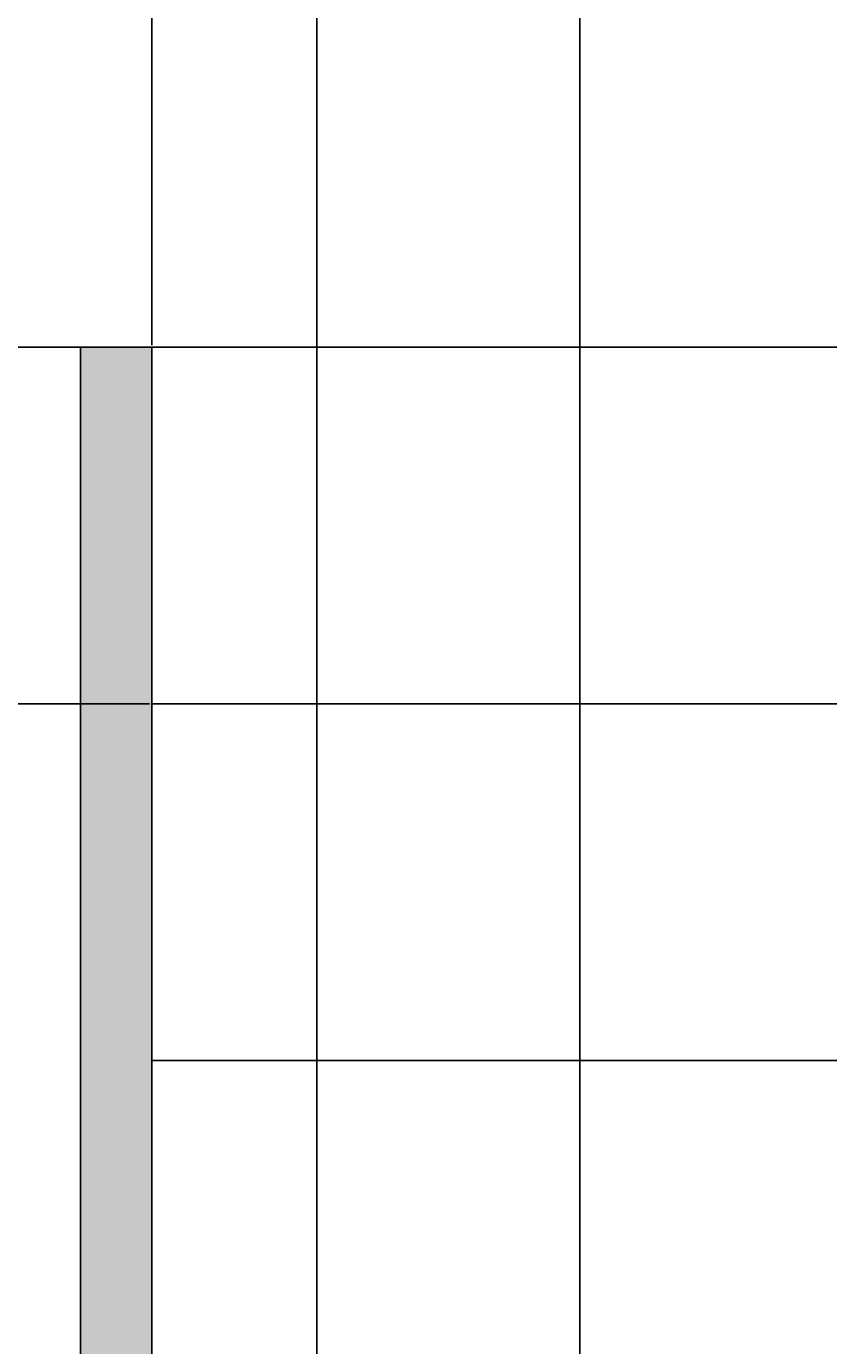
# Model space of a CAD drawing. Units: inches. Extents: x 2231 to 2461, y 2045 to 2455.
# Tile 62 of 95: x 2393 to 2416, y 2259 to 2296. Entities that reach past the tile are written whole.
import ezdxf

# ---------------------------------------------------------------- set-up
doc = ezdxf.new("R2010")
doc.units = ezdxf.units.IN
doc.layers.add('A-ANNO-DIMS', color=2, linetype='Continuous', lineweight=18)
doc.layers.add('A-FLOR-STRS', color=7, linetype='Continuous', lineweight=25)
doc.layers.add('A-WALL-PATT', color=18, linetype='Continuous', lineweight=13, true_color=0x000000)
doc.styles.get("Standard").update_dxf_attribs({"font": 'arial.ttf'})
doc.dimstyles.get("Standard").update_dxf_attribs({"dimtxt": 0.18, "dimasz": 0.18, "dimexe": 0.18, "dimexo": 0.0625, "dimgap": 0.09, "dimtad": 0, "dimtih": 1, "dimtoh": 1, "dimdec": 4, "dimzin": 0, "dimdsep": 46, "dimtxsty": 'Standard', "dimcen": 0.09, "dimadec": 0, "dimazin": 0, "dimtfac": 1, "dimtdec": 4, "dimtofl": 0, "dimtmove": 0, "dimatfit": 3, "dimfxl": 1, "dimtolj": 1, "dimtzin": 0, "dimarcsym": 0})

# ---------------------------------------------------------------- blocks, each defined once
blk = doc.blocks.new('*D42')
at = {"layer": 'A-ANNO-DIMS', "color": 0, "lineweight": -2, "transparency": 16777216}
for p, q in [((2396.794, 2286.895), (2396.794, 2454.645)), ((2432.794, 2286.895), (2432.794, 2454.645)), ((2396.974, 2454.465), (2414.575, 2454.465)), ((2432.614, 2454.465), (2415.012, 2454.465))]:
    blk.add_line(p, q, dxfattribs=at)
at = {"layer": 'A-ANNO-DIMS', "color": 0, "transparency": 16777216}
for points in [[(2396.974, 2454.495), (2396.974, 2454.435), (2396.794, 2454.465)], [(2432.614, 2454.495), (2432.614, 2454.435), (2432.794, 2454.465)]]:
    blk.add_solid(points, dxfattribs=at)
at = {"layer": 'Defpoints', "color": 0, "transparency": 16777216}
for p in [(2432.794, 2454.465), (2396.794, 2286.833), (2432.794, 2286.833)]:
    blk.add_point(p, dxfattribs=at)
at = {"layer": 'A-ANNO-DIMS', "color": 0, "transparency": 16777216, "insert": (2414.794, 2454.465), "char_height": 0.18, "attachment_point": 5}
blk.add_mtext('\\A1;36', dxfattribs=at)
blk = doc.blocks.new('*D59')
at = {"layer": 'A-ANNO-DIMS', "color": 0, "lineweight": -2, "transparency": 16777216}
for p, q in [((2408.794, 2182.895), (2408.794, 2454.645)), ((2432.794, 2182.895), (2432.794, 2454.645)), ((2408.974, 2454.465), (2420.573, 2454.465)), ((2432.614, 2454.465), (2421.014, 2454.465))]:
    blk.add_line(p, q, dxfattribs=at)
at = {"layer": 'A-ANNO-DIMS', "color": 0, "transparency": 16777216}
for points in [[(2408.974, 2454.495), (2408.974, 2454.435), (2408.794, 2454.465)], [(2432.614, 2454.495), (2432.614, 2454.435), (2432.794, 2454.465)]]:
    blk.add_solid(points, dxfattribs=at)
at = {"layer": 'Defpoints', "color": 0, "transparency": 16777216}
for p in [(2432.794, 2454.465), (2408.794, 2182.833), (2432.794, 2182.833)]:
    blk.add_point(p, dxfattribs=at)
at = {"layer": 'A-ANNO-DIMS', "color": 0, "transparency": 16777216, "insert": (2420.794, 2454.465), "char_height": 0.18, "attachment_point": 5}
blk.add_mtext('\\A1;24', dxfattribs=at)
blk = doc.blocks.new('*D66')
at = {"layer": 'A-ANNO-DIMS', "color": 0, "lineweight": -2, "transparency": 16777216}
for p, q in [((2348.189, 2096.895), (2348.189, 2454.645)), ((2408.794, 2096.895), (2408.794, 2454.645)), ((2348.369, 2454.465), (2378.167, 2454.465)), ((2408.614, 2454.465), (2378.815, 2454.465))]:
    blk.add_line(p, q, dxfattribs=at)
at = {"layer": 'A-ANNO-DIMS', "color": 0, "transparency": 16777216}
for points in [[(2348.369, 2454.495), (2348.369, 2454.435), (2348.189, 2454.465)], [(2408.614, 2454.495), (2408.614, 2454.435), (2408.794, 2454.465)]]:
    blk.add_solid(points, dxfattribs=at)
at = {"layer": 'Defpoints', "color": 0, "transparency": 16777216}
for p in [(2408.794, 2454.465), (2348.189, 2096.833), (2408.794, 2096.833)]:
    blk.add_point(p, dxfattribs=at)
at = {"layer": 'A-ANNO-DIMS', "color": 0, "transparency": 16777216, "insert": (2378.491, 2454.465), "char_height": 0.18, "attachment_point": 5}
blk.add_mtext('\\A1;60.6', dxfattribs=at)
blk = doc.blocks.new('*D71')
at = {"layer": 'A-ANNO-DIMS', "color": 0, "lineweight": -2, "transparency": 16777216}
for p, q in [((2401.422, 2092.979), (2401.422, 2454.645)), ((2408.794, 2096.895), (2408.794, 2454.645)), ((2401.602, 2454.465), (2404.732, 2454.465)), ((2408.614, 2454.465), (2405.483, 2454.465))]:
    blk.add_line(p, q, dxfattribs=at)
at = {"layer": 'A-ANNO-DIMS', "color": 0, "transparency": 16777216}
for points in [[(2401.602, 2454.495), (2401.602, 2454.435), (2401.422, 2454.465)], [(2408.614, 2454.495), (2408.614, 2454.435), (2408.794, 2454.465)]]:
    blk.add_solid(points, dxfattribs=at)
at = {"layer": 'Defpoints', "color": 0, "transparency": 16777216}
for p in [(2408.794, 2454.465), (2408.794, 2096.833), (2401.422, 2092.917)]:
    blk.add_point(p, dxfattribs=at)
at = {"layer": 'A-ANNO-DIMS', "color": 0, "transparency": 16777216, "insert": (2405.108, 2454.465), "char_height": 0.18, "attachment_point": 5}
blk.add_mtext('\\A1;7.371', dxfattribs=at)
blk = doc.blocks.new('*D72')
at = {"layer": 'A-ANNO-DIMS', "color": 0, "lineweight": -2, "transparency": 16777216}
for p, q in [((2384.543, 2145.12), (2384.543, 2454.645)), ((2408.794, 2150.677), (2408.794, 2454.645)), ((2384.723, 2454.465), (2396.272, 2454.465)), ((2408.614, 2454.465), (2397.064, 2454.465))]:
    blk.add_line(p, q, dxfattribs=at)
at = {"layer": 'A-ANNO-DIMS', "color": 0, "transparency": 16777216}
for points in [[(2384.723, 2454.495), (2384.723, 2454.435), (2384.543, 2454.465)], [(2408.614, 2454.495), (2408.614, 2454.435), (2408.794, 2454.465)]]:
    blk.add_solid(points, dxfattribs=at)
at = {"layer": 'Defpoints', "color": 0, "transparency": 16777216}
for p in [(2408.794, 2454.465), (2408.794, 2150.615), (2384.543, 2145.058)]:
    blk.add_point(p, dxfattribs=at)
at = {"layer": 'A-ANNO-DIMS', "color": 0, "transparency": 16777216, "insert": (2396.668, 2454.465), "char_height": 0.18, "attachment_point": 5}
blk.add_mtext('\\A1;24.25', dxfattribs=at)
blk = doc.blocks.new('*D74')
at = {"layer": 'A-ANNO-DIMS', "color": 0, "lineweight": -2, "transparency": 16777216}
for p, q in [((2396.731, 2286.833), (2377.981, 2286.833)), ((2378.161, 2286.653), (2378.161, 2282.015)), ((2378.161, 2277.013), (2378.161, 2281.651)), ((2396.731, 2276.833), (2377.981, 2276.833))]:
    blk.add_line(p, q, dxfattribs=at)
at = {"layer": 'A-ANNO-DIMS', "color": 0, "transparency": 16777216}
for points in [[(2378.131, 2286.653), (2378.191, 2286.653), (2378.161, 2286.833)], [(2378.131, 2277.013), (2378.191, 2277.013), (2378.161, 2276.833)]]:
    blk.add_solid(points, dxfattribs=at)
at = {"layer": 'Defpoints', "color": 0, "transparency": 16777216}
for p in [(2378.161, 2286.833), (2396.794, 2286.833), (2396.794, 2276.833)]:
    blk.add_point(p, dxfattribs=at)
at = {"layer": 'A-ANNO-DIMS', "color": 0, "transparency": 16777216, "insert": (2378.161, 2281.833), "char_height": 0.18, "attachment_point": 5}
blk.add_mtext('\\A1;10', dxfattribs=at)

msp = doc.modelspace()

# ---------------------------------------------------------------- hatches: boundary and pattern name
at = {"layer": 'A-WALL-PATT'}
h = msp.add_hatch(color=256, dxfattribs=at)
h.dxf.hatch_style = 1
h.paths.add_polyline_path([(2441.7935, 2269.1535), (2432.7935, 2269.1535), (2432.7935, 2186.8328), (2396.7935, 2186.8328), (2396.7935, 2286.8328), (2394.7935, 2286.8328), (2394.7935, 2186.8328), (2334.7935, 2186.8328), (2334.7935, 2182.8328), (2432.7935, 2182.8328), (2432.7935, 2072.8328), (2416.6639, 2072.8328), (2416.6639, 2063.8328), (2441.7935, 2063.8328)])
h.paths.add_polyline_path([(2368.6639, 2072.8328), (2367.04, 2072.8328), (2330.7942, 2072.8328), (2330.7397, 2063.8328), (2368.6639, 2063.8328)])
h.paths.add_polyline_path([(2300.7392, 2068.3328), (2300.7392, 2072.8328), (2298.7935, 2072.8328), (2294.7935, 2072.8328), (2258.7935, 2072.8328), (2258.7935, 2120.8328), (2294.7935, 2120.8328), (2298.7935, 2120.8328), (2298.7935, 2128.8328), (2294.7935, 2128.8328), (2294.7935, 2124.8328), (2258.7935, 2124.8328), (2258.7935, 2182.8328), (2294.7935, 2182.8328), (2294.7935, 2174.8328), (2298.7935, 2174.8328), (2298.7935, 2182.8328), (2304.7935, 2182.8328), (2304.7935, 2186.8328), (2258.7935, 2186.8328), (2258.7935, 2221.999), (2249.7935, 2221.999), (2249.7935, 2063.8328), (2300.7392, 2063.8328)])
h.paths.add_polyline_path([(2391.9338, 2435.8328), (2333.82, 2435.8328), (2333.82, 2426.8328), (2368.7935, 2426.8328), (2368.7935, 2374.9508), (2368.7935, 2370.8328), (2372.3935, 2370.8328), (2372.7935, 2370.8328), (2372.7935, 2426.8328), (2391.9338, 2426.8328)])
h.paths.add_polyline_path([(2441.7935, 2435.8328), (2415.9338, 2435.8328), (2415.9338, 2426.8328), (2432.7935, 2426.8328), (2432.7935, 2334.8328), (2372.7935, 2334.8328), (2372.7935, 2346.8328), (2368.7935, 2346.8328), (2368.7935, 2306.8328), (2360.7935, 2306.8328), (2360.7935, 2302.8328), (2368.7935, 2302.8328), (2372.7935, 2302.8328), (2372.7935, 2330.8328), (2432.7935, 2330.8328), (2432.7935, 2317.1535), (2441.7935, 2317.1535)])
h.paths.add_polyline_path([(2285.82, 2435.8328), (2249.7935, 2435.8328), (2249.7935, 2269.999), (2258.7935, 2269.999), (2258.7935, 2302.8328), (2318.8168, 2302.8328), (2330.7935, 2302.8328), (2330.7935, 2306.8328), (2258.7935, 2306.8328), (2258.7935, 2426.8328), (2285.82, 2426.8328)])

# ---------------------------------------------------------------- linework, layer by layer
at = {"layer": 'A-FLOR-STRS'}
for p, q in [((2394.7935, 2286.8328), (2394.7935, 2186.8328)), ((2394.7935, 2286.8328), (2432.7935, 2286.8328)), ((2396.7935, 2286.8328), (2396.7935, 2186.8328)), ((2396.7935, 2276.8328), (2432.7935, 2276.8328)), ((2396.7935, 2266.8328), (2432.7935, 2266.8328))]:
    msp.add_line(p, q, dxfattribs=at)

# ---------------------------------------------------------------- dimensions: what is measured, and where the dimension line sits
at = {"layer": 'A-ANNO-DIMS'}
for base, p1, p2, override, picture, middle in [((2408.7935, 2454.4653), (2348.1888, 2096.8328), (2408.7935, 2096.8328), {"dimdec": 1, "dimlfac": 1, "dimrnd": 0, "dimzin": 0, "dimdsep": 46, "dimlunit": 2}, '*D66', (2378.4912, 2454.4653)), ((2408.7935, 2454.4653), (2384.5428, 2145.0576), (2408.7935, 2150.6145), {"dimdec": 2, "dimlfac": 1, "dimrnd": 0, "dimzin": 0, "dimdsep": 46, "dimlunit": 2}, '*D72', (2396.6682, 2454.4653)), ((2432.7935, 2454.4653), (2396.7935, 2286.8328), (2432.7935, 2286.8328), {"dimdec": 0, "dimlfac": 1, "dimrnd": 0, "dimzin": 0, "dimdsep": 46, "dimlunit": 2}, '*D42', (2414.7935, 2454.4653)), ((2408.7935, 2454.4653), (2401.4221, 2092.9167), (2408.7935, 2096.8328), {"dimdec": 3, "dimlfac": 1, "dimrnd": 0, "dimzin": 0, "dimdsep": 46, "dimlunit": 2}, '*D71', (2405.1078, 2454.4653)), ((2432.7935, 2454.4653), (2408.7935, 2182.8328), (2432.7935, 2182.8328), {"dimdec": 0, "dimlfac": 1, "dimrnd": 0, "dimzin": 0, "dimdsep": 46, "dimlunit": 2}, '*D59', (2420.7935, 2454.4653))]:
    dim = msp.add_linear_dim(base=base, p1=p1, p2=p2, dimstyle='Standard', override=override, dxfattribs=at)
    dim.commit()
    dim.dimension.update_dxf_attribs({"geometry": picture, "text_midpoint": middle})
dim = msp.add_linear_dim(base=(2378.161, 2286.8328), p1=(2396.7935, 2276.8328), p2=(2396.7935, 2286.8328), angle=90, dimstyle='Standard', override={"dimdec": 0, "dimlfac": 1, "dimrnd": 0, "dimzin": 0, "dimdsep": 46, "dimlunit": 2}, dxfattribs=at)
dim.commit()
dim.dimension.update_dxf_attribs({"geometry": '*D74', "text_midpoint": (2378.161, 2281.8328)})

doc.saveas('drawing.dxf')
